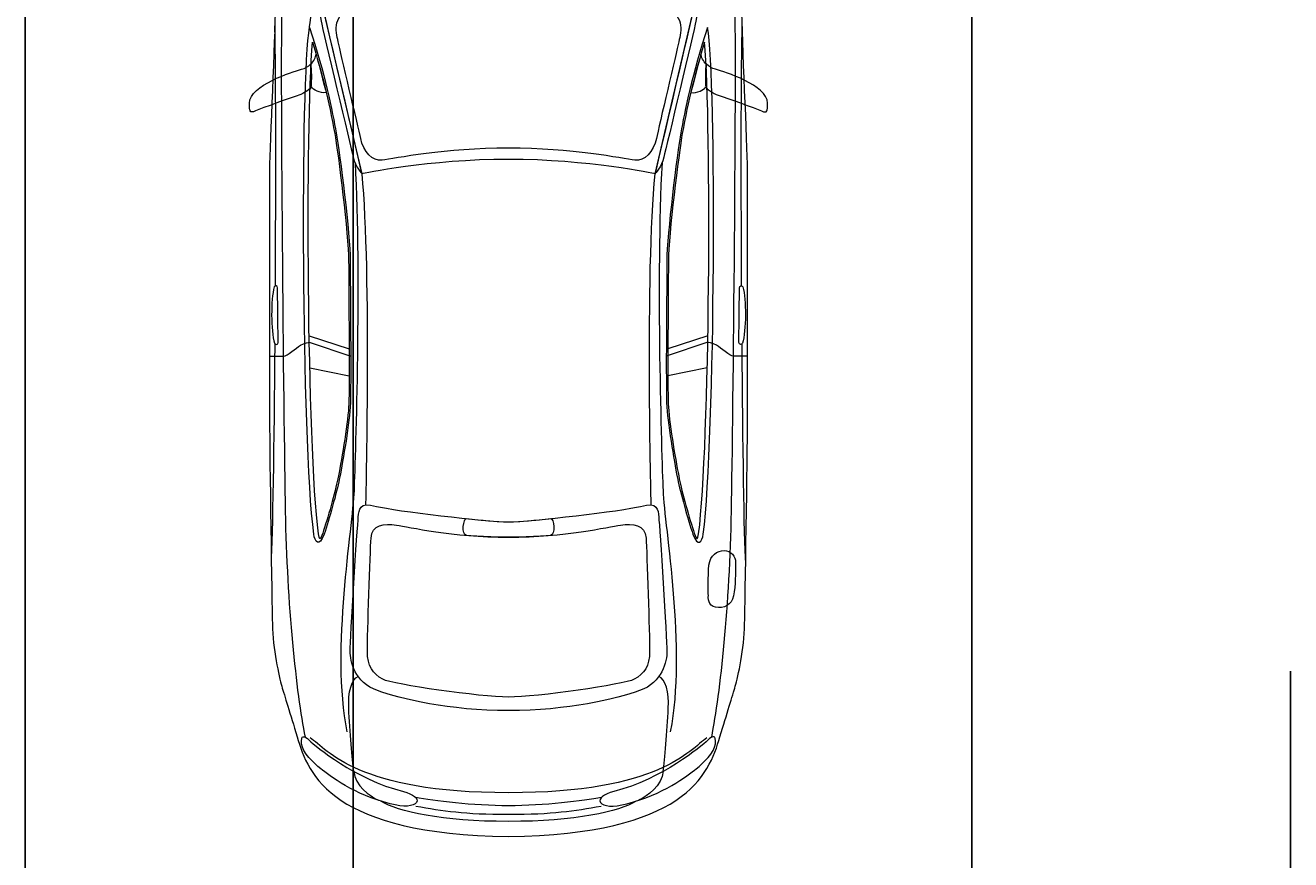
# Model space of a CAD drawing. Units: inches. Extents: x 1734 to 2405, y 1500 to 2491.
# Tile 4 of 14: x 1798 to 1900, y 1784 to 1851. Entities that reach past the tile are written whole.
import ezdxf

# ---------------------------------------------------------------- set-up
doc = ezdxf.new("R2010")
doc.units = ezdxf.units.IN
for name, color, linetype, lineweight in [('A-ANNO-DIMS', 2, 'Continuous', 18), ('AUDI', 8, 'Continuous', 18), ('C-PROP', 7, 'Continuous', 25)]:
    doc.layers.add(name, color=color, linetype=linetype, lineweight=lineweight)
doc.styles.get("Standard").update_dxf_attribs({"font": 'arial.ttf'})
doc.dimstyles.get("Standard").update_dxf_attribs({"dimtxt": 0.18, "dimasz": 0.18, "dimexe": 0.18, "dimexo": 0.0625, "dimgap": 0.09, "dimtad": 0, "dimtih": 1, "dimtoh": 1, "dimdec": 4, "dimzin": 0, "dimdsep": 46, "dimtxsty": 'Standard', "dimcen": 0.09, "dimadec": 0, "dimazin": 0, "dimtfac": 1, "dimtdec": 4, "dimtofl": 0, "dimtmove": 0, "dimatfit": 3, "dimfxl": 1, "dimtolj": 1, "dimtzin": 0, "dimarcsym": 0})

# ---------------------------------------------------------------- blocks, each defined once
blk = doc.blocks.new('*D26')
at = {"layer": 'A-ANNO-DIMS', "color": 0, "lineweight": -2, "transparency": 16777216}
for p, q in [((1900.39, 1798.76), (1900.39, 1615.47)), ((1932.99, 1798.76), (1932.99, 1615.47)), ((1900.57, 1615.65), (1916.37, 1615.65)), ((1932.81, 1615.65), (1917.02, 1615.65))]:
    blk.add_line(p, q, dxfattribs=at)
at = {"layer": 'A-ANNO-DIMS', "color": 0, "transparency": 16777216}
for points in [[(1900.57, 1615.68), (1900.57, 1615.62), (1900.39, 1615.65)], [(1932.81, 1615.68), (1932.81, 1615.62), (1932.99, 1615.65)]]:
    blk.add_solid(points, dxfattribs=at)
at = {"layer": 'Defpoints', "color": 0, "transparency": 16777216}
for p in [(1900.39, 1798.82), (1932.99, 1798.82), (1932.99, 1615.65)]:
    blk.add_point(p, dxfattribs=at)
at = {"layer": 'A-ANNO-DIMS', "color": 0, "transparency": 16777216, "insert": (1916.69, 1615.65), "char_height": 0.18, "attachment_point": 5}
blk.add_mtext('\\A1;32.6', dxfattribs=at)
blk = doc.blocks.new('*D32')
at = {"layer": 'A-ANNO-DIMS', "color": 0, "lineweight": -2, "transparency": 16777216}
for p, q in [((1798.39, 2202.26), (1798.39, 1615.47)), ((1824.83, 2202.26), (1824.83, 1615.47)), ((1798.57, 1615.65), (1811.22, 1615.65)), ((1824.65, 1615.65), (1812.01, 1615.65))]:
    blk.add_line(p, q, dxfattribs=at)
at = {"layer": 'A-ANNO-DIMS', "color": 0, "transparency": 16777216}
for points in [[(1798.57, 1615.68), (1798.57, 1615.62), (1798.39, 1615.65)], [(1824.65, 1615.68), (1824.65, 1615.62), (1824.83, 1615.65)]]:
    blk.add_solid(points, dxfattribs=at)
at = {"layer": 'Defpoints', "color": 0, "transparency": 16777216}
for p in [(1798.39, 2202.32), (1824.83, 2202.32), (1824.83, 1615.65)]:
    blk.add_point(p, dxfattribs=at)
at = {"layer": 'A-ANNO-DIMS', "color": 0, "transparency": 16777216, "insert": (1811.61, 1615.65), "char_height": 0.18, "attachment_point": 5}
blk.add_mtext('\\A1;26.44', dxfattribs=at)
blk = doc.blocks.new('*D33')
at = {"layer": 'A-ANNO-DIMS', "color": 0, "lineweight": -2, "transparency": 16777216}
for p, q in [((1824.83, 2202.26), (1824.83, 1615.47)), ((1874.68, 2202.26), (1874.68, 1615.47)), ((1825.01, 1615.65), (1849.36, 1615.65)), ((1874.5, 1615.65), (1850.15, 1615.65))]:
    blk.add_line(p, q, dxfattribs=at)
at = {"layer": 'A-ANNO-DIMS', "color": 0, "transparency": 16777216}
for points in [[(1825.01, 1615.68), (1825.01, 1615.62), (1824.83, 1615.65)], [(1874.5, 1615.68), (1874.5, 1615.62), (1874.68, 1615.65)]]:
    blk.add_solid(points, dxfattribs=at)
at = {"layer": 'Defpoints', "color": 0, "transparency": 16777216}
for p in [(1824.83, 2202.32), (1874.68, 2202.32), (1874.68, 1615.65)]:
    blk.add_point(p, dxfattribs=at)
at = {"layer": 'A-ANNO-DIMS', "color": 0, "transparency": 16777216, "insert": (1849.76, 1615.65), "char_height": 0.18, "attachment_point": 5}
blk.add_mtext('\\A1;49.84', dxfattribs=at)

msp = doc.modelspace()

# ---------------------------------------------------------------- linework, layer by layer
at = {"layer": 'AUDI'}
for points, knots in [([(1837.345, 1785.4381), (1823.2241, 1785.5924), (1821.1737, 1790.3408), (1820.3073, 1793.4695), (1820.3073, 1793.4695), (1819.7422, 1795.3167), (1819.2902, 1796.7867), (1819.0641, 1797.5407), (1819.0641, 1797.5407), (1818.838, 1798.2946), (1818.3485, 1800.5941), (1818.3107, 1802.5166), (1818.3107, 1802.5166), (1818.2728, 1804.4391), (1818.0863, 1815.9017), (1818.0863, 1819.0652), (1818.0863, 1819.0652), (1818.0863, 1822.2286), (1818.0863, 1837.0491), (1818.0863, 1839.1573), (1818.0863, 1839.1573), (1818.0863, 1841.2655), (1818.5368, 1849.6746), (1818.5368, 1852.3509), (1818.5368, 1852.3509), (1818.5368, 1855.0274), (1818.0863, 1858.3854), (1818.0863, 1859.7768), (1818.0863, 1859.7768), (1818.0863, 1861.1684), (1818.3482, 1868.5223), (1818.4614, 1870.1433), (1818.4614, 1870.1433), (1818.5745, 1871.7643), (1819.1815, 1872.6836), (1819.7048, 1873.8376), (1819.7048, 1873.8376), (1821.7393, 1878.3231), (1826.9383, 1880.7733), (1827.5035, 1881.1503), (1827.5035, 1881.1503), (1828.0686, 1881.5274), (1828.6686, 1881.7322), (1829.3873, 1881.7322), (1829.3873, 1881.7322), (1830.1059, 1881.7322), (1830.2914, 1881.3766), (1830.5929, 1881.452), (1830.5929, 1881.452), (1830.8943, 1881.5274), (1831.6453, 1881.7322), (1832.4769, 1881.7322), (1832.4769, 1881.7322), (1833.3085, 1881.7322), (1837.345, 1881.7322), (1837.345, 1881.7322), (1837.345, 1881.7322), (1837.345, 1881.7322), (1841.3816, 1881.7322), (1842.2132, 1881.7322), (1842.2132, 1881.7322), (1843.0448, 1881.7322), (1843.7957, 1881.5274), (1844.0972, 1881.452), (1844.0972, 1881.452), (1844.3986, 1881.3766), (1844.5842, 1881.7322), (1845.3028, 1881.7322), (1845.3028, 1881.7322), (1846.0215, 1881.7322), (1846.6215, 1881.5274), (1847.1866, 1881.1503), (1847.1866, 1881.1503), (1847.7517, 1880.7733), (1852.9508, 1878.3231), (1854.9853, 1873.8376), (1854.9853, 1873.8376), (1855.5085, 1872.6836), (1856.1155, 1871.7643), (1856.2287, 1870.1433), (1856.2287, 1870.1433), (1856.3419, 1868.5224), (1856.6038, 1861.1684), (1856.6038, 1859.7768), (1856.6038, 1859.7768), (1856.6038, 1858.3854), (1856.1533, 1855.0274), (1856.1533, 1852.3509), (1856.1533, 1852.3509), (1856.1533, 1849.6746), (1856.6038, 1841.2655), (1856.6038, 1839.1573), (1856.6038, 1839.1573), (1856.6038, 1837.0491), (1856.6038, 1822.2286), (1856.6038, 1819.0652), (1856.6038, 1819.0652), (1856.6038, 1815.9017), (1856.4172, 1804.4391), (1856.3794, 1802.5166), (1856.3794, 1802.5166), (1856.3417, 1800.5941), (1855.8521, 1798.2946), (1855.626, 1797.5407), (1855.626, 1797.5407), (1855.3998, 1796.7867), (1854.9479, 1795.3166), (1854.3827, 1793.4695), (1854.3827, 1793.4695), (1853.5163, 1790.3408), (1851.466, 1785.5924), (1837.345, 1785.4381)], [0, 0, 0, 0, 0.03571429, 0.03571429, 0.03571429, 0.0357143, 0.07142857, 0.07142857, 0.07142857, 0.07142858, 0.10714286, 0.10714286, 0.10714286, 0.10714287, 0.14285714, 0.14285714, 0.14285714, 0.14285715, 0.17857143, 0.17857143, 0.17857143, 0.17857144, 0.21428571, 0.21428571, 0.21428571, 0.21428572, 0.25, 0.25, 0.25, 0.25000001, 0.28571429, 0.28571429, 0.28571429, 0.2857143, 0.32142857, 0.32142857, 0.32142857, 0.32142858, 0.35714286, 0.35714286, 0.35714286, 0.35714287, 0.39285714, 0.39285714, 0.39285714, 0.39285715, 0.42857143, 0.42857143, 0.42857143, 0.42857144, 0.46428571, 0.46428571, 0.46428571, 0.46428572, 0.5, 0.5, 0.5, 0.50000001, 0.53571429, 0.53571429, 0.53571429, 0.5357143, 0.57142857, 0.57142857, 0.57142857, 0.57142858, 0.60714286, 0.60714286, 0.60714286, 0.60714287, 0.64285714, 0.64285714, 0.64285714, 0.64285715, 0.67857143, 0.67857143, 0.67857143, 0.67857144, 0.71428571, 0.71428571, 0.71428571, 0.71428572, 0.75, 0.75, 0.75, 0.75000001, 0.78571429, 0.78571429, 0.78571429, 0.7857143, 0.82142857, 0.82142857, 0.82142857, 0.82142858, 0.85714286, 0.85714286, 0.85714286, 0.85714287, 0.89285714, 0.89285714, 0.89285714, 0.89285715, 0.92857143, 0.92857143, 0.92857143, 0.92857144, 0.96428571, 0.96428571, 0.96428571, 0.96428572, 1, 1, 1, 1]), ([(1820.9696, 1793.4282), (1820.2601, 1796.9777), (1819.5047, 1804.1661), (1819.3757, 1811.6524), (1819.3757, 1811.6524), (1819.2466, 1819.1387), (1818.9243, 1847.9218), (1819.1178, 1853.9881), (1819.1178, 1853.9881), (1819.3112, 1860.0545), (1819.4195, 1867.7073), (1820.4941, 1872.916)], [0, 0, 0, 0, 0.33333333, 0.33333333, 0.33333333, 0.33333334, 0.66666667, 0.66666667, 0.66666667, 0.66666668, 1, 1, 1, 1]), ([(1853.7205, 1793.4282), (1854.43, 1796.9777), (1855.1854, 1804.1661), (1855.3144, 1811.6524), (1855.3144, 1811.6524), (1855.4435, 1819.1387), (1855.7658, 1847.9218), (1855.5723, 1853.9881), (1855.5723, 1853.9881), (1855.3788, 1860.0545), (1855.2706, 1867.7073), (1854.1959, 1872.916)], [0, 0, 0, 0, 0.33333333, 0.33333333, 0.33333333, 0.33333334, 0.66666667, 0.66666667, 0.66666667, 0.66666668, 1, 1, 1, 1]), ([(1837.345, 1839.9913), (1843.7369, 1839.9913), (1849.1528, 1838.8351), (1849.1528, 1838.8351), (1849.1528, 1838.8351), (1849.1528, 1838.8351), (1852.5232, 1853.1904), (1852.5232, 1853.1904), (1852.5232, 1853.1904), (1851.175, 1854.0577), (1849.4184, 1856.9963), (1837.345, 1856.9963), (1837.345, 1856.9963), (1825.2717, 1856.9963), (1823.515, 1854.0577), (1822.1669, 1853.1904), (1822.1669, 1853.1904), (1822.1669, 1853.1904), (1825.5373, 1838.8351), (1825.5373, 1838.8351), (1825.5373, 1838.8351), (1825.5373, 1838.8351), (1830.9532, 1839.9913), (1837.345, 1839.9913)], [0, 0, 0, 0, 0.16666667, 0.16666667, 0.16666667, 0.16666668, 0.33333333, 0.33333333, 0.33333333, 0.33333334, 0.5, 0.5, 0.5, 0.50000001, 0.66666667, 0.66666667, 0.66666667, 0.66666668, 0.83333333, 0.83333333, 0.83333333, 0.83333334, 1, 1, 1, 1]), ([(1837.345, 1839.9913), (1843.7369, 1839.9913), (1849.1528, 1838.8351), (1849.1528, 1838.8351), (1849.1528, 1838.8351), (1849.1528, 1838.8351), (1852.5232, 1853.1904), (1852.5232, 1853.1904), (1852.5232, 1853.1904), (1851.175, 1854.0577), (1849.4184, 1856.9963), (1837.345, 1856.9963), (1837.345, 1856.9963), (1825.2717, 1856.9963), (1823.515, 1854.0577), (1822.1669, 1853.1904), (1822.1669, 1853.1904), (1822.1669, 1853.1904), (1825.5373, 1838.8351), (1825.5373, 1838.8351), (1825.5373, 1838.8351), (1825.5373, 1838.8351), (1830.9532, 1839.9913), (1837.345, 1839.9913)], [0, 0, 0, 0, 0.16666667, 0.16666667, 0.16666667, 0.16666668, 0.33333333, 0.33333333, 0.33333333, 0.33333334, 0.5, 0.5, 0.5, 0.50000001, 0.66666667, 0.66666667, 0.66666667, 0.66666668, 0.83333333, 0.83333333, 0.83333333, 0.83333334, 1, 1, 1, 1]), ([(1837.345, 1840.8946), (1842.4186, 1840.8946), (1846.5714, 1840.0626), (1847.5327, 1839.9172), (1847.5327, 1839.9172), (1848.3171, 1839.7985), (1849.0424, 1840.6471), (1849.2623, 1841.6646), (1849.2623, 1841.6646), (1849.4821, 1842.682), (1850.8838, 1848.6218), (1851.0763, 1849.4743), (1851.0763, 1849.4743), (1851.2687, 1850.3268), (1851.5984, 1851.7292), (1849.7295, 1852.3066), (1849.7295, 1852.3066), (1847.8606, 1852.8843), (1844.5569, 1854.0665), (1837.345, 1854.0665), (1837.345, 1854.0665), (1830.1332, 1854.0665), (1826.8295, 1852.8842), (1824.9606, 1852.3066), (1824.9606, 1852.3066), (1823.0916, 1851.7293), (1823.4214, 1850.3267), (1823.6138, 1849.4743), (1823.6138, 1849.4743), (1823.8062, 1848.6218), (1825.2079, 1842.682), (1825.4278, 1841.6646), (1825.4278, 1841.6646), (1825.6477, 1840.6471), (1826.373, 1839.7985), (1827.1574, 1839.9172), (1827.1574, 1839.9172), (1828.1187, 1840.0626), (1832.2714, 1840.8946), (1837.345, 1840.8946)], [0, 0, 0, 0, 0.1, 0.1, 0.1, 0.10000001, 0.2, 0.2, 0.2, 0.20000001, 0.3, 0.3, 0.3, 0.30000001, 0.4, 0.4, 0.4, 0.40000001, 0.5, 0.5, 0.5, 0.50000001, 0.6, 0.6, 0.6, 0.60000001, 0.7, 0.7, 0.7, 0.70000001, 0.8, 0.8, 0.8, 0.80000001, 0.9, 0.9, 0.9, 0.90000001, 1, 1, 1, 1]), ([(1822.1668, 1853.1904), (1822.1668, 1853.1904), (1825.5373, 1838.8351), (1825.5373, 1838.8351), (1825.5373, 1838.8351), (1825.5373, 1838.8351), (1825.0104, 1839.3572), (1824.8178, 1840.1762), (1824.8178, 1840.1762), (1824.6251, 1840.9952), (1822.3895, 1850.352), (1822.245, 1851.1227), (1822.245, 1851.1227), (1822.1005, 1851.8934), (1822.1669, 1853.1904), (1822.1668, 1853.1904)], [0, 0, 0, 0, 0.25, 0.25, 0.25, 0.25000001, 0.5, 0.5, 0.5, 0.50000001, 0.75, 0.75, 0.75, 0.75000001, 1, 1, 1, 1]), ([(1822.1668, 1853.1904), (1822.1668, 1853.1904), (1825.5373, 1838.8351), (1825.5373, 1838.8351), (1825.5373, 1838.8351), (1825.5373, 1838.8351), (1825.0104, 1839.3572), (1824.8178, 1840.1762), (1824.8178, 1840.1762), (1824.6251, 1840.9952), (1822.3895, 1850.352), (1822.245, 1851.1227), (1822.245, 1851.1227), (1822.1005, 1851.8934), (1822.1668, 1853.1904), (1822.1668, 1853.1904)], [0, 0, 0, 0, 0.25, 0.25, 0.25, 0.25000001, 0.5, 0.5, 0.5, 0.50000001, 0.75, 0.75, 0.75, 0.75000001, 1, 1, 1, 1]), ([(1852.5232, 1853.1904), (1852.5232, 1853.1904), (1849.1528, 1838.8351), (1849.1528, 1838.8351), (1849.1528, 1838.8351), (1849.1528, 1838.8351), (1849.6797, 1839.3572), (1849.8723, 1840.1762), (1849.8723, 1840.1762), (1850.0649, 1840.9952), (1852.3006, 1850.352), (1852.4451, 1851.1227), (1852.4451, 1851.1227), (1852.5896, 1851.8934), (1852.5232, 1853.1904), (1852.5232, 1853.1904)], [0, 0, 0, 0, 0.25, 0.25, 0.25, 0.25000001, 0.5, 0.5, 0.5, 0.50000001, 0.75, 0.75, 0.75, 0.75000001, 1, 1, 1, 1]), ([(1821.6474, 1809.7879), (1821.7226, 1809.1974), (1822.0878, 1808.6623), (1822.4791, 1809.7879), (1822.4791, 1809.7879), (1822.8703, 1810.9134), (1823.5061, 1813.2133), (1823.7017, 1814.1919), (1823.7017, 1814.1919), (1823.8972, 1815.1704), (1824.4843, 1818.3999), (1824.582, 1820.0147), (1824.582, 1820.0147), (1824.6797, 1821.6295), (1824.582, 1829.8991), (1824.582, 1831.8563), (1824.582, 1831.8563), (1824.582, 1833.8138), (1823.7506, 1840.5176), (1823.4571, 1842.1323), (1823.4571, 1842.1323), (1823.1636, 1843.747), (1822.5278, 1846.9766), (1821.3035, 1850.6144), (1821.3035, 1850.6144), (1820.5717, 1846.5852), (1820.6692, 1817.4702), (1821.6474, 1809.7879)], [0, 0, 0, 0, 0.14285714, 0.14285714, 0.14285714, 0.14285715, 0.28571429, 0.28571429, 0.28571429, 0.2857143, 0.42857143, 0.42857143, 0.42857143, 0.42857144, 0.57142857, 0.57142857, 0.57142857, 0.57142858, 0.71428571, 0.71428571, 0.71428571, 0.71428572, 0.85714286, 0.85714286, 0.85714286, 0.85714287, 1, 1, 1, 1]), ([(1853.0427, 1809.7879), (1852.9675, 1809.1974), (1852.6023, 1808.6623), (1852.211, 1809.7879), (1852.211, 1809.7879), (1851.8198, 1810.9134), (1851.1841, 1813.2133), (1850.9884, 1814.1919), (1850.9884, 1814.1919), (1850.7929, 1815.1704), (1850.2057, 1818.3999), (1850.1081, 1820.0147), (1850.1081, 1820.0147), (1850.0103, 1821.6295), (1850.1081, 1829.8991), (1850.1081, 1831.8563), (1850.1081, 1831.8563), (1850.1081, 1833.8138), (1850.9394, 1840.5176), (1851.233, 1842.1323), (1851.233, 1842.1323), (1851.5265, 1843.747), (1852.1623, 1846.9766), (1853.3866, 1850.6144), (1853.3866, 1850.6144), (1854.1184, 1846.5852), (1854.0209, 1817.4702), (1853.0427, 1809.7879)], [0, 0, 0, 0, 0.14285714, 0.14285714, 0.14285714, 0.14285715, 0.28571429, 0.28571429, 0.28571429, 0.2857143, 0.42857143, 0.42857143, 0.42857143, 0.42857144, 0.57142857, 0.57142857, 0.57142857, 0.57142858, 0.71428571, 0.71428571, 0.71428571, 0.71428572, 0.85714286, 0.85714286, 0.85714286, 0.85714287, 1, 1, 1, 1]), ([(1822.0193, 1809.8193), (1822.0193, 1809.8193), (1822.0193, 1809.8193), (1822.0193, 1809.8193), (1822.0193, 1809.8193), (1822.0468, 1809.6031), (1822.1057, 1809.4776), (1822.1484, 1809.4171), (1822.1484, 1809.4171), (1822.193, 1809.4704), (1822.2701, 1809.588), (1822.3681, 1809.8698), (1822.3681, 1809.8698), (1822.7494, 1810.9667), (1823.3845, 1813.2543), (1823.5816, 1814.2407), (1823.5816, 1814.2407), (1823.8178, 1815.4224), (1824.3664, 1818.5204), (1824.4577, 1820.0297), (1824.4577, 1820.0297), (1824.5292, 1821.2106), (1824.4948, 1826.0362), (1824.4723, 1829.2294), (1824.4723, 1829.2294), (1824.4723, 1829.2294), (1824.4572, 1831.8564), (1824.4572, 1831.8564), (1824.4572, 1831.8564), (1824.4572, 1833.8082), (1823.6168, 1840.5442), (1823.3364, 1842.0876), (1823.3364, 1842.0876), (1822.8672, 1844.6686), (1822.2587, 1847.1263), (1821.539, 1849.4311), (1821.539, 1849.4311), (1820.964, 1842.7543), (1821.1127, 1816.9377), (1822.0193, 1809.8193)], [0, 0, 0, 0, 0.1, 0.1, 0.1, 0.10000001, 0.2, 0.2, 0.2, 0.20000001, 0.3, 0.3, 0.3, 0.30000001, 0.4, 0.4, 0.4, 0.40000001, 0.5, 0.5, 0.5, 0.50000001, 0.6, 0.6, 0.6, 0.60000001, 0.7, 0.7, 0.7, 0.70000001, 0.8, 0.8, 0.8, 0.80000001, 0.9, 0.9, 0.9, 0.90000001, 1, 1, 1, 1]), ([(1852.6708, 1809.8193), (1852.6708, 1809.8193), (1852.6708, 1809.8193), (1852.6708, 1809.8193), (1852.6708, 1809.8193), (1852.6433, 1809.6031), (1852.5844, 1809.4776), (1852.5417, 1809.4171), (1852.5417, 1809.4171), (1852.497, 1809.4704), (1852.42, 1809.588), (1852.322, 1809.8698), (1852.322, 1809.8698), (1851.9407, 1810.9667), (1851.3056, 1813.2543), (1851.1085, 1814.2407), (1851.1085, 1814.2407), (1850.8723, 1815.4224), (1850.3237, 1818.5204), (1850.2324, 1820.0297), (1850.2324, 1820.0297), (1850.1609, 1821.2106), (1850.1953, 1826.0362), (1850.2178, 1829.2294), (1850.2178, 1829.2294), (1850.2178, 1829.2294), (1850.2328, 1831.8564), (1850.2328, 1831.8564), (1850.2328, 1831.8564), (1850.2328, 1833.8082), (1851.0733, 1840.5442), (1851.3537, 1842.0876), (1851.3537, 1842.0876), (1851.8228, 1844.6686), (1852.4314, 1847.1263), (1853.1511, 1849.4311), (1853.1511, 1849.4311), (1853.7261, 1842.7543), (1853.5773, 1816.9377), (1852.6708, 1809.8193)], [0, 0, 0, 0, 0.1, 0.1, 0.1, 0.10000001, 0.2, 0.2, 0.2, 0.20000001, 0.3, 0.3, 0.3, 0.30000001, 0.4, 0.4, 0.4, 0.40000001, 0.5, 0.5, 0.5, 0.50000001, 0.6, 0.6, 0.6, 0.60000001, 0.7, 0.7, 0.7, 0.70000001, 0.8, 0.8, 0.8, 0.80000001, 0.9, 0.9, 0.9, 0.90000001, 1, 1, 1, 1]), ([(1821.385, 1847.6526), (1821.4628, 1847.2502), (1821.4699, 1846.3739), (1821.4228, 1845.7707), (1821.4228, 1845.7707), (1821.4402, 1845.7899), (1821.4595, 1845.8094), (1821.4714, 1845.8265), (1821.4714, 1845.8265), (1821.5796, 1845.5968), (1822.1366, 1845.2936), (1822.6486, 1845.3776), (1822.6486, 1845.3776), (1822.5815, 1845.6585), (1821.8334, 1848.4584), (1821.8334, 1848.4584), (1821.8334, 1848.4584), (1821.8029, 1848.2267), (1821.6571, 1847.9122), (1821.385, 1847.6526)], [0, 0, 0, 0, 0.2, 0.2, 0.2, 0.20000001, 0.4, 0.4, 0.4, 0.40000001, 0.6, 0.6, 0.6, 0.60000001, 0.8, 0.8, 0.8, 0.80000001, 1, 1, 1, 1]), ([(1853.3051, 1847.6526), (1853.2273, 1847.2502), (1853.2202, 1846.3739), (1853.2673, 1845.7707), (1853.2673, 1845.7707), (1853.2499, 1845.7899), (1853.2306, 1845.8094), (1853.2187, 1845.8265), (1853.2187, 1845.8265), (1853.1105, 1845.5968), (1852.5535, 1845.2936), (1852.0414, 1845.3776), (1852.0414, 1845.3776), (1852.1086, 1845.6585), (1852.8567, 1848.4584), (1852.8567, 1848.4584), (1852.8567, 1848.4584), (1852.8872, 1848.2267), (1853.033, 1847.9122), (1853.3051, 1847.6526)], [0, 0, 0, 0, 0.2, 0.2, 0.2, 0.20000001, 0.4, 0.4, 0.4, 0.40000001, 0.6, 0.6, 0.6, 0.60000001, 0.8, 0.8, 0.8, 0.80000001, 1, 1, 1, 1]), ([(1821.385, 1847.6526), (1821.2025, 1847.4783), (1820.9646, 1847.3281), (1820.6606, 1847.2465), (1820.6606, 1847.2465), (1819.9037, 1847.0434), (1816.4982, 1845.9756), (1816.4576, 1844.5151), (1816.4576, 1844.5151), (1816.4576, 1843.893), (1816.471, 1843.6768), (1816.9575, 1843.893), (1816.9575, 1843.893), (1817.4441, 1844.1094), (1819.8904, 1844.9881), (1820.2958, 1845.1098), (1820.2958, 1845.1098), (1820.669, 1845.2222), (1821.2207, 1845.5502), (1821.4228, 1845.7707), (1821.4228, 1845.7707), (1821.4699, 1846.3739), (1821.4628, 1847.2502), (1821.385, 1847.6526)], [0, 0, 0, 0, 0.16666667, 0.16666667, 0.16666667, 0.16666668, 0.33333333, 0.33333333, 0.33333333, 0.33333334, 0.5, 0.5, 0.5, 0.50000001, 0.66666667, 0.66666667, 0.66666667, 0.66666668, 0.83333333, 0.83333333, 0.83333333, 0.83333334, 1, 1, 1, 1]), ([(1853.3051, 1847.6526), (1853.4875, 1847.4783), (1853.7254, 1847.3281), (1854.0295, 1847.2465), (1854.0295, 1847.2465), (1854.7864, 1847.0434), (1858.1919, 1845.9756), (1858.2325, 1844.5151), (1858.2325, 1844.5151), (1858.2325, 1843.893), (1858.2191, 1843.6768), (1857.7326, 1843.893), (1857.7326, 1843.893), (1857.246, 1844.1094), (1854.7997, 1844.9881), (1854.3943, 1845.1098), (1854.3943, 1845.1098), (1854.0211, 1845.2222), (1853.4693, 1845.5502), (1853.2673, 1845.7707), (1853.2673, 1845.7707), (1853.2202, 1846.3739), (1853.2273, 1847.2502), (1853.3051, 1847.6526)], [0, 0, 0, 0, 0.16666667, 0.16666667, 0.16666667, 0.16666668, 0.33333333, 0.33333333, 0.33333333, 0.33333334, 0.5, 0.5, 0.5, 0.50000001, 0.66666667, 0.66666667, 0.66666667, 0.66666668, 0.83333333, 0.83333333, 0.83333333, 0.83333334, 1, 1, 1, 1]), ([(1824.9713, 1839.7129), (1825.4774, 1830.5798), (1825.0012, 1816.2172), (1824.8912, 1813.3023), (1824.8912, 1813.3023), (1824.7813, 1810.3875), (1822.9972, 1800.4872), (1824.3046, 1793.8628)], [0, 0, 0, 0, 0.5, 0.5, 0.5, 0.50000001, 1, 1, 1, 1]), ([(1849.7188, 1839.7129), (1849.2127, 1830.5798), (1849.6889, 1816.2172), (1849.7989, 1813.3023), (1849.7989, 1813.3023), (1849.9088, 1810.3875), (1851.6929, 1800.4872), (1850.3855, 1793.8628)], [0, 0, 0, 0, 0.5, 0.5, 0.5, 0.50000001, 1, 1, 1, 1]), ([(1818.7764, 1825.2407), (1818.7764, 1825.0682), (1818.5404, 1825.0033), (1818.488, 1825.1761), (1818.488, 1825.1761), (1818.3304, 1825.6724), (1818.2523, 1826.557), (1818.2523, 1827.4417), (1818.2523, 1827.4417), (1818.2523, 1828.3264), (1818.3044, 1829.1894), (1818.4616, 1829.7073), (1818.4616, 1829.7073), (1818.514, 1829.8584), (1818.7236, 1829.8151), (1818.7236, 1829.6425), (1818.7236, 1829.6425), (1818.7236, 1829.6425), (1818.7764, 1825.2407), (1818.7764, 1825.2407)], [0, 0, 0, 0, 0.2, 0.2, 0.2, 0.20000001, 0.4, 0.4, 0.4, 0.40000001, 0.6, 0.6, 0.6, 0.60000001, 0.8, 0.8, 0.8, 0.80000001, 1, 1, 1, 1]), ([(1855.9137, 1825.2407), (1855.9137, 1825.0682), (1856.1496, 1825.0033), (1856.2021, 1825.1761), (1856.2021, 1825.1761), (1856.3597, 1825.6724), (1856.4378, 1826.557), (1856.4378, 1827.4417), (1856.4378, 1827.4417), (1856.4378, 1828.3264), (1856.3857, 1829.1894), (1856.2285, 1829.7073), (1856.2285, 1829.7073), (1856.1761, 1829.8584), (1855.9665, 1829.8151), (1855.9665, 1829.6425), (1855.9665, 1829.6425), (1855.9665, 1829.6425), (1855.9137, 1825.2407), (1855.9137, 1825.2407)], [0, 0, 0, 0, 0.2, 0.2, 0.2, 0.20000001, 0.4, 0.4, 0.4, 0.40000001, 0.6, 0.6, 0.6, 0.60000001, 0.8, 0.8, 0.8, 0.80000001, 1, 1, 1, 1]), ([(1818.0863, 1824.1326), (1818.0863, 1824.1326), (1818.9349, 1824.1325), (1819.2136, 1824.1325), (1819.2136, 1824.1325), (1819.4922, 1824.1325), (1820.2309, 1824.8084), (1820.5717, 1825.0059), (1820.5717, 1825.0059), (1820.9124, 1825.2035), (1821.2867, 1825.2503), (1821.2867, 1825.2503)], [0, 0, 0, 0, 0.33333333, 0.33333333, 0.33333333, 0.33333334, 0.66666667, 0.66666667, 0.66666667, 0.66666668, 1, 1, 1, 1]), ([(1856.6038, 1824.1326), (1856.6038, 1824.1326), (1855.7552, 1824.1325), (1855.4765, 1824.1325), (1855.4765, 1824.1325), (1855.1978, 1824.1325), (1854.4592, 1824.8084), (1854.1184, 1825.0059), (1854.1184, 1825.0059), (1853.7777, 1825.2035), (1853.4034, 1825.2503), (1853.4034, 1825.2503)], [0, 0, 0, 0, 0.33333333, 0.33333333, 0.33333333, 0.33333334, 0.66666667, 0.66666667, 0.66666667, 0.66666668, 1, 1, 1, 1]), ([(1837.345, 1795.5674), (1842.0925, 1795.5674), (1846.0833, 1796.5206), (1847.9155, 1797.1806), (1847.9155, 1797.1806), (1849.7478, 1797.8406), (1850.1143, 1799.5272), (1850.1143, 1800.3704), (1850.1143, 1800.3704), (1850.1143, 1801.2138), (1849.5279, 1810.49), (1849.4546, 1811.1501), (1849.4546, 1811.1501), (1849.3815, 1811.81), (1849.4179, 1812.3967), (1847.9888, 1812.03), (1847.9888, 1812.03), (1846.5596, 1811.6633), (1839.1206, 1810.7834), (1837.345, 1810.7834), (1837.345, 1810.7834), (1835.5695, 1810.7835), (1828.1305, 1811.6633), (1826.7013, 1812.03), (1826.7013, 1812.03), (1825.2721, 1812.3967), (1825.3086, 1811.81), (1825.2354, 1811.1501), (1825.2354, 1811.1501), (1825.1622, 1810.49), (1824.5758, 1801.2137), (1824.5758, 1800.3704), (1824.5758, 1800.3704), (1824.5758, 1799.5272), (1824.9423, 1797.8406), (1826.7745, 1797.1806), (1826.7745, 1797.1806), (1828.6067, 1796.5206), (1832.5975, 1795.5674), (1837.345, 1795.5674)], [0, 0, 0, 0, 0.1, 0.1, 0.1, 0.10000001, 0.2, 0.2, 0.2, 0.20000001, 0.3, 0.3, 0.3, 0.30000001, 0.4, 0.4, 0.4, 0.40000001, 0.5, 0.5, 0.5, 0.50000001, 0.6, 0.6, 0.6, 0.60000001, 0.7, 0.7, 0.7, 0.70000001, 0.8, 0.8, 0.8, 0.80000001, 0.9, 0.9, 0.9, 0.90000001, 1, 1, 1, 1]), ([(1837.345, 1795.5674), (1842.0925, 1795.5674), (1846.0833, 1796.5206), (1847.9155, 1797.1806), (1847.9155, 1797.1806), (1849.7478, 1797.8406), (1850.1143, 1799.5272), (1850.1143, 1800.3704), (1850.1143, 1800.3704), (1850.1143, 1801.2138), (1849.5279, 1810.49), (1849.4546, 1811.1501), (1849.4546, 1811.1501), (1849.3815, 1811.81), (1849.4179, 1812.3967), (1847.9888, 1812.03), (1847.9888, 1812.03), (1846.5596, 1811.6633), (1839.1206, 1810.7834), (1837.345, 1810.7834), (1837.345, 1810.7834), (1835.5695, 1810.7834), (1828.1305, 1811.6633), (1826.7013, 1812.03), (1826.7013, 1812.03), (1825.2721, 1812.3967), (1825.3086, 1811.81), (1825.2354, 1811.1501), (1825.2354, 1811.1501), (1825.1622, 1810.49), (1824.5758, 1801.2137), (1824.5758, 1800.3704), (1824.5758, 1800.3704), (1824.5758, 1799.5272), (1824.9423, 1797.8406), (1826.7745, 1797.1806), (1826.7745, 1797.1806), (1828.6067, 1796.5206), (1832.5975, 1795.5674), (1837.345, 1795.5674)], [0, 0, 0, 0, 0.1, 0.1, 0.1, 0.10000001, 0.2, 0.2, 0.2, 0.20000001, 0.3, 0.3, 0.3, 0.30000001, 0.4, 0.4, 0.4, 0.40000001, 0.5, 0.5, 0.5, 0.50000001, 0.6, 0.6, 0.6, 0.60000001, 0.7, 0.7, 0.7, 0.70000001, 0.8, 0.8, 0.8, 0.80000001, 0.9, 0.9, 0.9, 0.90000001, 1, 1, 1, 1]), ([(1837.345, 1796.665), (1839.597, 1796.665), (1846.6695, 1797.6573), (1847.4758, 1798.0973), (1847.4758, 1798.0973), (1848.2821, 1798.5372), (1848.7218, 1799.1605), (1848.7218, 1800.3704), (1848.7218, 1800.3704), (1848.7218, 1801.5804), (1848.5017, 1808.3635), (1848.4285, 1809.4634), (1848.4285, 1809.4634), (1848.3553, 1810.5635), (1847.3659, 1810.6735), (1846.3765, 1810.5267), (1846.3765, 1810.5267), (1845.387, 1810.3801), (1841.9057, 1809.5369), (1837.345, 1809.5369), (1837.345, 1809.5369), (1832.7843, 1809.5369), (1829.3031, 1810.3801), (1828.3136, 1810.5267), (1828.3136, 1810.5267), (1827.3242, 1810.6735), (1826.3348, 1810.5635), (1826.2615, 1809.4634), (1826.2615, 1809.4634), (1826.1883, 1808.3636), (1825.9682, 1801.5804), (1825.9682, 1800.3704), (1825.9682, 1800.3704), (1825.9682, 1799.1605), (1826.408, 1798.5372), (1827.2143, 1798.0973), (1827.2143, 1798.0973), (1828.0205, 1797.6574), (1835.093, 1796.665), (1837.345, 1796.665)], [0, 0, 0, 0, 0.1, 0.1, 0.1, 0.10000001, 0.2, 0.2, 0.2, 0.20000001, 0.3, 0.3, 0.3, 0.30000001, 0.4, 0.4, 0.4, 0.40000001, 0.5, 0.5, 0.5, 0.50000001, 0.6, 0.6, 0.6, 0.60000001, 0.7, 0.7, 0.7, 0.70000001, 0.8, 0.8, 0.8, 0.80000001, 0.9, 0.9, 0.9, 0.90000001, 1, 1, 1, 1]), ([(1837.345, 1809.5369), (1837.345, 1809.5369), (1840.034, 1809.5841), (1840.7353, 1809.6875), (1840.7353, 1809.6875), (1841.1739, 1809.7523), (1840.9676, 1811.0641), (1840.7626, 1811.0442), (1840.7626, 1811.0442), (1839.474, 1810.9192), (1838.3905, 1810.7834), (1837.345, 1810.7834), (1837.345, 1810.7834), (1836.2995, 1810.7834), (1835.2161, 1810.9192), (1833.9276, 1811.0442), (1833.9276, 1811.0442), (1833.7225, 1811.0641), (1833.5162, 1809.7522), (1833.9548, 1809.6875), (1833.9548, 1809.6875), (1834.6561, 1809.5841), (1837.345, 1809.5369), (1837.345, 1809.5369)], [0, 0, 0, 0, 0.16666667, 0.16666667, 0.16666667, 0.16666668, 0.33333333, 0.33333333, 0.33333333, 0.33333334, 0.5, 0.5, 0.5, 0.50000001, 0.66666667, 0.66666667, 0.66666667, 0.66666668, 0.83333333, 0.83333333, 0.83333333, 0.83333334, 1, 1, 1, 1]), ([(1853.4532, 1804.8636), (1853.4023, 1804.3844), (1853.5739, 1803.8876), (1854.2691, 1803.8744), (1854.2691, 1803.8744), (1854.9644, 1803.861), (1855.442, 1804.2313), (1855.5439, 1805.1497), (1855.5439, 1805.1497), (1855.6459, 1806.068), (1855.6459, 1806.9862), (1855.6459, 1807.4965), (1855.6459, 1807.4965), (1855.6459, 1808.0067), (1855.2888, 1808.4657), (1854.728, 1808.4657), (1854.728, 1808.4657), (1854.1672, 1808.4657), (1853.6063, 1808.1088), (1853.5043, 1807.2925), (1853.5043, 1807.2925), (1853.4023, 1806.4761), (1853.4532, 1804.8636), (1853.4532, 1804.8636)], [0, 0, 0, 0, 0.16666667, 0.16666667, 0.16666667, 0.16666668, 0.33333333, 0.33333333, 0.33333333, 0.33333334, 0.5, 0.5, 0.5, 0.50000001, 0.66666667, 0.66666667, 0.66666667, 0.66666668, 0.83333333, 0.83333333, 0.83333333, 0.83333334, 1, 1, 1, 1]), ([(1824.8695, 1790.677), (1824.7613, 1791.5814), (1824.5472, 1793.8958), (1824.4658, 1795.769), (1824.4658, 1795.769), (1824.4109, 1797.034), (1824.6823, 1798.1615), (1825.2337, 1798.3127)], [0, 0, 0, 0, 0.5, 0.5, 0.5, 0.50000001, 1, 1, 1, 1]), ([(1849.8206, 1790.677), (1849.9288, 1791.5814), (1850.1428, 1793.8958), (1850.2242, 1795.769), (1850.2242, 1795.769), (1850.2792, 1797.034), (1850.0078, 1798.1615), (1849.4564, 1798.3127)], [0, 0, 0, 0, 0.5, 0.5, 0.5, 0.50000001, 1, 1, 1, 1]), ([(1828.868, 1789.0458), (1824.953, 1790.0584), (1821.7823, 1792.6973), (1821.2934, 1793.172), (1821.2934, 1793.172), (1820.8631, 1793.5899), (1820.5987, 1793.6357), (1820.6659, 1792.8997), (1820.6659, 1792.8997), (1820.7323, 1792.1735), (1821.6479, 1791.3554), (1822.2098, 1790.8893), (1822.2098, 1790.8893), (1822.9276, 1790.2939), (1824.8981, 1788.8075), (1827.8093, 1788.0662), (1827.8093, 1788.0662), (1828.9209, 1787.7484), (1829.7149, 1787.8543), (1829.9266, 1788.172), (1829.9266, 1788.172), (1830.1384, 1788.4898), (1829.6456, 1788.8437), (1828.868, 1789.0458)], [0, 0, 0, 0, 0.16666667, 0.16666667, 0.16666667, 0.16666668, 0.33333333, 0.33333333, 0.33333333, 0.33333334, 0.5, 0.5, 0.5, 0.50000001, 0.66666667, 0.66666667, 0.66666667, 0.66666668, 0.83333333, 0.83333333, 0.83333333, 0.83333334, 1, 1, 1, 1]), ([(1853.3293, 1793.3756), (1851.9283, 1792.4141), (1849.5315, 1788.9493), (1837.345, 1788.9493), (1837.345, 1788.9493), (1825.1585, 1788.9493), (1822.7618, 1792.4141), (1821.3608, 1793.3756)], [0, 0, 0, 0, 0.5, 0.5, 0.5, 0.50000001, 1, 1, 1, 1]), ([(1845.822, 1789.0458), (1849.737, 1790.0584), (1852.9078, 1792.6973), (1853.3967, 1793.172), (1853.3967, 1793.172), (1853.827, 1793.5899), (1854.0914, 1793.6357), (1854.0241, 1792.8997), (1854.0241, 1792.8997), (1853.9578, 1792.1735), (1853.0422, 1791.3554), (1852.4803, 1790.8893), (1852.4803, 1790.8893), (1851.7625, 1790.2939), (1849.792, 1788.8075), (1846.8808, 1788.0662), (1846.8808, 1788.0662), (1845.7692, 1787.7484), (1844.9752, 1787.8543), (1844.7634, 1788.172), (1844.7634, 1788.172), (1844.5517, 1788.4898), (1845.0445, 1788.8437), (1845.822, 1789.0458)], [0, 0, 0, 0, 0.16666667, 0.16666667, 0.16666667, 0.16666668, 0.33333333, 0.33333333, 0.33333333, 0.33333334, 0.5, 0.5, 0.5, 0.50000001, 0.66666667, 0.66666667, 0.66666667, 0.66666668, 0.83333333, 0.83333333, 0.83333333, 0.83333334, 1, 1, 1, 1]), ([(1847.6272, 1788.2784), (1846.2665, 1787.4096), (1842.7154, 1786.6396), (1837.345, 1786.6396), (1837.345, 1786.6396), (1831.9746, 1786.6396), (1828.4236, 1787.4096), (1827.0629, 1788.2784)], [0, 0, 0, 0, 0.5, 0.5, 0.5, 0.50000001, 1, 1, 1, 1]), ([(1844.8223, 1788.5586), (1843.4081, 1788.2894), (1840.1869, 1787.9044), (1837.345, 1787.9044), (1837.345, 1787.9044), (1834.5032, 1787.9044), (1831.2819, 1788.2894), (1829.8678, 1788.5586)], [0, 0, 0, 0, 0.5, 0.5, 0.5, 0.50000001, 1, 1, 1, 1]), ([(1844.8223, 1787.8494), (1842.6385, 1787.4645), (1840.9014, 1787.1895), (1837.345, 1787.1895), (1837.345, 1787.1895), (1833.7886, 1787.1895), (1832.0515, 1787.4645), (1829.8678, 1787.8494)], [0, 0, 0, 0, 0.5, 0.5, 0.5, 0.50000001, 1, 1, 1, 1])]:
    msp.add_open_spline(points, degree=3, knots=knots, dxfattribs=at)
for points in [[(1821.2776, 1850.3817), (1821.3509, 1851.0418), (1821.5068, 1852.6837), (1822.1669, 1853.1904)], [(1818.5537, 1829.7944), (1818.602, 1838.5422), (1818.5965, 1847.2409), (1818.5078, 1850.7432)], [(1856.1364, 1829.7944), (1856.0881, 1838.5422), (1856.0937, 1847.2409), (1856.1823, 1850.7432)], [(1825.8465, 1812.1366), (1825.8465, 1812.1366), (1826.3157, 1830.8448), (1825.5373, 1838.8351)], [(1848.8436, 1812.1366), (1848.8436, 1812.1366), (1848.3744, 1830.8448), (1849.1528, 1838.8351)], [(1818.2284, 1807.4263), (1818.3536, 1809.6599), (1818.4599, 1816.9982), (1818.5228, 1825.1147)], [(1821.2772, 1825.7834), (1821.2772, 1825.7834), (1824.4983, 1824.7259), (1824.4983, 1824.7259)], [(1821.2867, 1825.2503), (1821.2867, 1825.2503), (1824.6245, 1824.1326), (1824.6245, 1824.1326)], [(1853.4034, 1825.2503), (1853.4034, 1825.2503), (1850.0656, 1824.1326), (1850.0656, 1824.1326)], [(1853.4129, 1825.7834), (1853.4129, 1825.7834), (1850.1918, 1824.7259), (1850.1918, 1824.7259)], [(1856.4616, 1807.4263), (1856.3365, 1809.6599), (1856.2302, 1816.9982), (1856.1673, 1825.1147)], [(1821.3292, 1823.1926), (1821.3292, 1823.1926), (1824.4996, 1822.559), (1824.4996, 1822.559)], [(1853.3608, 1823.1926), (1853.3608, 1823.1926), (1850.1905, 1822.559), (1850.1905, 1822.559)], [(1824.8695, 1790.677), (1824.993, 1789.5186), (1826.1291, 1788.6924), (1826.8682, 1788.3409)], [(1849.8206, 1790.677), (1849.6971, 1789.5186), (1848.561, 1788.6924), (1847.8219, 1788.3409)]]:
    msp.add_open_spline(points, degree=3, dxfattribs=at)
at = {"layer": 'C-PROP'}
msp.add_line((1798.3942, 1900.8246), (1798.3942, 1710.7667), dxfattribs=at)

# ---------------------------------------------------------------- dimensions: what is measured, and where the dimension line sits
at = {"layer": 'A-ANNO-DIMS'}
for base, p1, p2, override, picture, middle in [((1824.8343, 1615.6468), (1798.3942, 2202.3246), (1824.8343, 2202.3246), {"dimdec": 2, "dimlfac": 1, "dimrnd": 0, "dimzin": 0, "dimdsep": 46, "dimlunit": 2}, '*D32', (1811.6142, 1615.6468)), ((1874.676, 1615.6468), (1824.8343, 2202.3246), (1874.676, 2202.3246), {"dimdec": 2, "dimlfac": 1, "dimrnd": 0, "dimzin": 0, "dimdsep": 46, "dimlunit": 2}, '*D33', (1849.7551, 1615.6468)), ((1932.9923, 1615.6468), (1900.3942, 1798.8246), (1932.9923, 1798.8246), {"dimdec": 1, "dimlfac": 1, "dimrnd": 0, "dimzin": 0, "dimdsep": 46, "dimlunit": 2}, '*D26', (1916.6932, 1615.6468))]:
    dim = msp.add_linear_dim(base=base, p1=p1, p2=p2, dimstyle='Standard', override=override, dxfattribs=at)
    dim.commit()
    dim.dimension.update_dxf_attribs({"geometry": picture, "text_midpoint": middle})

doc.saveas('drawing.dxf')
